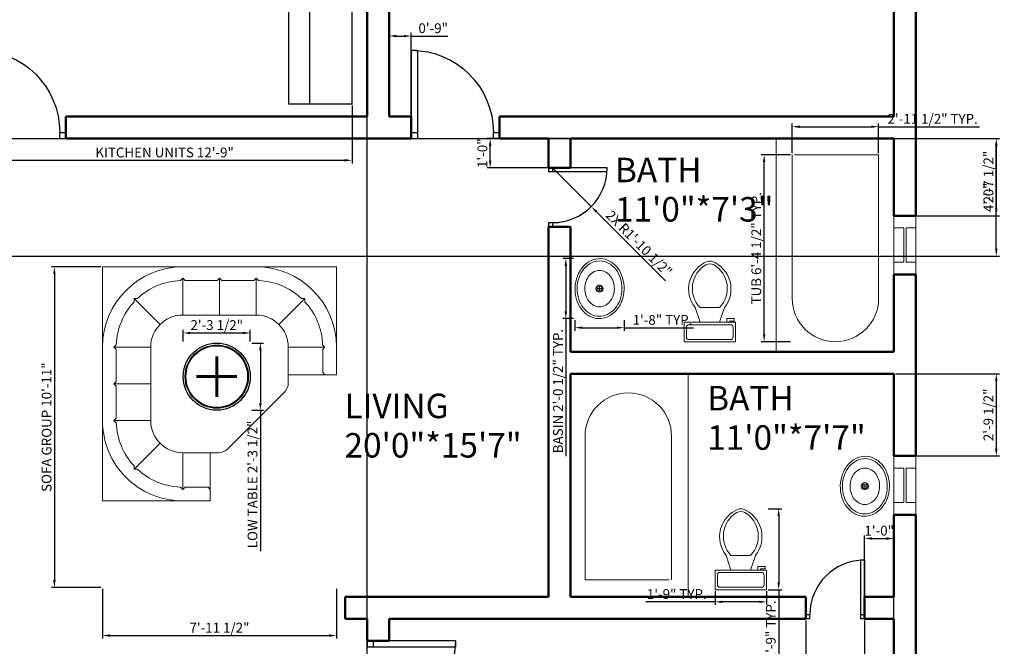
# Model space of a CAD drawing. Units: inches. Extents: x 2201 to 2875, y 1361 to 2074.
# Tile 3 of 4: x 2474 to 2875, y 1600 to 1855. Entities that reach past the tile are written whole.
import ezdxf

# ---------------------------------------------------------------- set-up
doc = ezdxf.new("R2010")
doc.units = ezdxf.units.IN
for name, color, linetype, lineweight in [('A-ANNO-DIMS', 2, 'Continuous', 18), ('A-AREA-IDEN', 7, 'Continuous', 25), ('A-FLOR-FIXT', 9, 'Continuous', 18), ('doors', 5, 'Continuous', 25), ('furniture', 8, 'Continuous', 18), ('ventilator', 3, 'Continuous', 18), ('walls', 6, 'Continuous', 50)]:
    doc.layers.add(name, color=color, linetype=linetype, lineweight=lineweight)
doc.layers.add('TEFRIŞ', color=11, linetype='Continuous')
doc.styles.get("Standard").update_dxf_attribs({"font": 'arial.ttf'})
doc.dimstyles.new('ISO-25', dxfattribs={"dimtxt": 4, "dimasz": 3, "dimexe": 1.25, "dimexo": 0.625, "dimtad": 1, "dimlunit": 3, "dimtxsty": 'Standard', "dimcen": 2.5, "dimadec": 0, "dimazin": 0, "dimtfac": 1, "dimtmove": 0, "dimatfit": 3, "dimfxl": 1, "dimarcsym": 0})

# ---------------------------------------------------------------- blocks, each defined once
blk = doc.blocks.new('12PRST09')
at = {"color": 0, "linetype": 'ByBlock'}
for p, q in [((47, 102), (0, 102)), ((0, 102), (0, 0)), ((47, 102), (47, 81)), ((35, 97), (33.98, 95.98)), ((36, 96), (35, 97)), ((35, 81), (35, 97)), ((36, 96), (46, 96)), ((46, 96), (47, 97)), ((15.23, 88.21), (13.79, 88.21)), ((13.79, 88.21), (13.79, 86.77)), ((25.1, 76.9), (13.79, 88.21)), ((50.51, 81), (35, 81)), ((54.76, 79.24), (79.24, 54.76)), ((5, 67), (6.02, 68.02)), ((6, 66), (5, 67)), ((21, 67), (5, 67)), ((6, 52), (6, 66)), ((21, 67), (21, 35)), ((5, 51), (6, 52)), ((6, 50), (5, 51)), ((21, 51), (5, 51)), ((6, 36), (6, 50)), ((81, 35), (81, 50.51)), ((102, 47), (81, 47)), ((96, 46), (97, 47)), ((96, 36), (96, 46)), ((102, 0), (102, 47)), ((6, 36), (5, 35)), ((21, 35), (5, 35)), ((5, 35), (6.02, 33.98)), ((81, 35), (97, 35)), ((97, 35), (95.98, 33.98)), ((96, 36), (97, 35)), ((25.1, 25.1), (13.79, 13.79)), ((76.9, 25.1), (88.21, 13.79)), ((35, 21), (35, 5)), ((35, 21), (67, 21)), ((51, 21), (51, 5)), ((67, 21), (67, 5)), ((13.79, 13.79), (13.79, 15.23)), ((15.23, 13.79), (13.79, 13.79)), ((86.77, 13.79), (88.21, 13.79)), ((88.21, 13.79), (88.21, 15.23)), ((35, 5), (33.98, 6.02)), ((36, 6), (35, 5)), ((50, 6), (36, 6)), ((50, 6), (51, 5)), ((51, 5), (52, 6)), ((66, 6), (52, 6)), ((66, 6), (67, 5)), ((67, 5), (68.02, 6.02)), ((0, 0), (102, 0))]:
    blk.add_line(p, q, dxfattribs=at)
for centre, radius, start, end in [((35, 67), 35, 90, 180), ((35, 67), 29, 92.0114, 132.9886), ((35, 67), 29, 137.0114, 177.9886), ((35, 67), 14, 90, 180), ((50.51, 75), 6, 45, 90), ((75, 50.51), 6, 0, 45), ((35, 35), 35, 180, 270), ((35, 35), 14, 180, 270), ((67, 35), 14, 270, 0), ((67, 35), 35, 270, 0), ((35, 35), 29, 182.0114, 222.9886), ((67, 35), 29, 317.0114, 357.9886), ((35, 35), 29, 227.0114, 267.9886), ((67, 35), 29, 272.0114, 312.9886)]:
    blk.add_arc(centre, radius, start, end, dxfattribs=at)
for tag, p, flags in [('ITEM', (75, 96), 3), ('ROOM_NUMBER', (74, 86), 1), ('DEPTH', (75, 74), 3), ('WIDTH', (75, 65), 3)]:
    blk.add_attdef(tag, p, '', height=6, dxfattribs=dict(at, flags=flags))
blk = doc.blocks.new('31')
at = {"layer": 'TEFRIŞ'}
for p, q in [((-1268.3, -203.6), (-1268.3, -264.3)), ((-1268.3, -264.3), (-1268.3, -203.6)), ((-1268.3, -264.3), (-1268.3, -203.6)), ((-1268.3, -203.6), (-1268.3, -264.3)), ((-1267.3, -203.6), (-1267.3, -264.3)), ((-1267.3, -264.3), (-1267.3, -203.6)), ((-1267.3, -264.3), (-1267.3, -203.6)), ((-1267.3, -203.6), (-1267.3, -264.3)), ((-1266.3, -203.6), (-1266.3, -264.3)), ((-1266.3, -264.3), (-1266.3, -203.6)), ((-1266.3, -264.3), (-1266.3, -203.6)), ((-1266.3, -203.6), (-1266.3, -264.3)), ((-1297.6, -232.9), (-1237, -232.9)), ((-1237, -232.9), (-1297.6, -232.9)), ((-1237, -232.9), (-1297.6, -232.9)), ((-1297.6, -232.9), (-1237, -232.9)), ((-1297.6, -233.9), (-1237, -233.9)), ((-1237, -233.9), (-1297.6, -233.9)), ((-1237, -233.9), (-1297.6, -233.9)), ((-1297.6, -233.9), (-1237, -233.9)), ((-1297.6, -234.9), (-1237, -234.9)), ((-1237, -234.9), (-1297.6, -234.9)), ((-1237, -234.9), (-1297.6, -234.9)), ((-1297.6, -234.9), (-1237, -234.9))]:
    blk.add_line(p, q, dxfattribs=at)
for radius in [50.3, 47.3, 46.3]:
    blk.add_circle((-1267.3, -233.9), radius, dxfattribs=at)
blk = doc.blocks.new('A$C008029BD')
at = {"layer": 'TEFRIŞ', "ltscale": 0.05}
for p, q in [((0, 0), (0, -3.55)), ((3.3699, 0), (0, 0)), ((3.3699, 0), (3.3699, -0.6)), ((1.5225, -0.4), (0, -0.4)), ((3.3699, -0.4), (2.0825, -0.4)), ((0.05, -0.5806), (0.05, -1.8694)), ((0.05, -0.5806), (0.55, -0.5806)), ((0.096, -0.6166), (0.454, -0.6166)), ((0.55, -0.5806), (0.55, -1.8694)), ((0.6, -2.71), (0.6, -0.6)), ((3.3699, -0.6), (0.6, -0.6)), ((0.086, -1.7734), (0.086, -0.6766)), ((0.0991, -0.6595), (0.4571, -0.6595)), ((0.1131, -0.954), (0.1131, -0.6955)), ((0.4931, -0.6955), (0.4931, -0.954)), ((0.514, -0.6766), (0.514, -1.7734)), ((0.2301, -0.8457), (0.2288, -0.9671)), ((0.2801, -0.8455), (0.2768, -1.1584)), ((0.096, -1.0242), (0.454, -1.0242)), ((0.4571, -0.99), (0.0991, -0.99)), ((0.2282, -1.0198), (0.2268, -1.1586)), ((0.11, -1.3187), (0.11, -1.0602)), ((0.49, -1.0602), (0.49, -1.3187)), ((0.454, -1.3547), (0.096, -1.3547)), ((0.096, -1.3912), (0.454, -1.3912)), ((0.11, -1.7734), (0.11, -1.4272)), ((0.1544, -1.7734), (0.1544, -1.4272)), ((0.2144, -1.7734), (0.2144, -1.4272)), ((0.2744, -1.7734), (0.2744, -1.4272)), ((0.3344, -1.7734), (0.3344, -1.4272)), ((0.3902, -1.7734), (0.3902, -1.4272)), ((0.4444, -1.7734), (0.4444, -1.4272)), ((0.49, -1.4272), (0.49, -1.7734)), ((0.454, -1.8094), (0.096, -1.8094)), ((0.454, -1.8334), (0.096, -1.8334)), ((0.55, -1.8694), (0.05, -1.8694)), ((0, -2.025), (0.4, -2.025)), ((0.4, -2.71), (0.4, -2.025)), ((0, -2.71), (0.6, -2.71)), ((0, -3.55), (0.65, -3.55))]:
    blk.add_line(p, q, dxfattribs=at)
at = {"layer": 'TEFRIŞ'}
blk.add_line((1.9688, -0.05), (1.9688, -0.5719), dxfattribs=at)
at = {"layer": 'TEFRIŞ', "ltscale": 0.05}
for points in [[(1.5225, -0.05), (2.0825, -0.05), (2.0825, -0.5719), (1.5225, -0.5719)], [(0.67, -2.73), (0.67, -3.53), (0.07, -3.53), (0.07, -2.73)], [(0.72, -2.78), (0.72, -3.48), (0.67, -3.48), (0.67, -2.78)]]:
    blk.add_lwpolyline(points, close=True, dxfattribs=at)
at = {"layer": 'TEFRIŞ', "const_width": 0.025}
for points in [[(2.0136, -0.1231, 1), (2.0386, -0.1231, 1)], [(2.0136, -0.2361, 1), (2.0386, -0.2361, 1)], [(2.0136, -0.3269, 1), (2.0386, -0.3269, 1)], [(2.0136, -0.4399, 1), (2.0386, -0.4399, 1)]]:
    blk.add_lwpolyline(points, format="xyb", close=True, dxfattribs=at)
at = {"layer": 'TEFRIŞ', "ltscale": 0.05}
for centre, radius in [((1.6277, -0.1636), 0.0505), ((1.6277, -0.4499), 0.0505), ((0.255, -0.8197), 0.036), ((0.2519, -1.1844), 0.036)]:
    blk.add_circle(centre, radius, dxfattribs=at)
at = {"layer": 'TEFRIŞ'}
for centre in [(1.8804, -0.1636), (1.8804, -0.4499)]:
    blk.add_circle(centre, 0.0505, dxfattribs=at)
at = {"layer": 'TEFRIŞ', "ltscale": 0.05}
for centre, radius, start, end in [((0.1083, -0.6495), 0.0351, 110.49764, 230.57771), ((0.454, -0.6766), 0.06, 0, 90), ((0.1177, -0.673), 0.023, 143.98534, 258.51568), ((0.4571, -0.6955), 0.036, 0, 90), ((0.1146, -1.0377), 0.023, 143.98534, 258.51568), ((0.1177, -0.9765), 0.023, 101.48432, 216.01466), ((0.454, -1.0602), 0.036, 0, 90), ((0.4571, -0.954), 0.036, 270, 0), ((0.1146, -1.3412), 0.023, 101.48432, 216.01466), ((0.1146, -1.4047), 0.023, 143.98534, 258.51568), ((0.454, -1.3187), 0.036, 270, 0), ((0.454, -1.4272), 0.036, 0, 90), ((0.1083, -1.8005), 0.0351, 129.42229, 249.50236), ((0.1146, -1.7959), 0.023, 101.48432, 216.01466), ((0.454, -1.7734), 0.06, 270, 0), ((0.454, -1.7734), 0.036, 270, 0)]:
    blk.add_arc(centre, radius, start, end, dxfattribs=at)
blk = doc.blocks.new('Sink - Oval top')
for p, q in [((-1, 0), (1, 0)), ((0, 1), (0, -1))]:
    blk.add_line(p, q)
for points in [[(-12.23, 0.39, 0.117634), (-11.46, -3.36, 0.104469), (-8.88, -6.8, 0.090016), (-5.08, -9.07, 0.08192), (-0.32, -10.02, 0.08192), (4.49, -9.38, 0.090016), (8.42, -7.36, 0.104469), (11.22, -4.09, 0.117634), (12.23, -0.39, 0.117634), (11.46, 3.36, 0.104469), (8.88, 6.8, 0.090016), (5.08, 9.07, 0.08192), (0.32, 10.02, 0.08192), (-4.49, 9.38, 0.090016), (-8.42, 7.36, 0.104469), (-11.22, 4.09, 0.117634)], [(-11.29, 0.16, 0.118622), (-10.52, -3.25, 0.104678), (-8.07, -6.36, 0.089562), (-4.54, -8.37, 0.081185), (-0.13, -9.15, 0.081185), (4.3, -8.49, 0.089562), (7.89, -6.58, 0.104678), (10.42, -3.55, 0.118622), (11.29, -0.16, 0.118622), (10.52, 3.25, 0.104678), (8.07, 6.36, 0.089562), (4.54, 8.37, 0.081185), (0.13, 9.15, 0.081185), (-4.3, 8.49, 0.089562), (-7.89, 6.58, 0.104678), (-10.42, 3.55, 0.118622)], [(-7.42, 0.08, 0.118283), (-6.91, -2.17, 0.104607), (-5.29, -4.21, 0.089718), (-2.97, -5.53, 0.081436), (-0.07, -6.04, 0.081436), (2.84, -5.59, 0.089718), (5.2, -4.33, 0.104607), (6.86, -2.32, 0.118283), (7.42, -0.08, 0.118283), (6.91, 2.17, 0.104607), (5.29, 4.21, 0.089718), (2.97, 5.53, 0.081436), (0.07, 6.04, 0.081436), (-2.84, 5.59, 0.089718), (-5.2, 4.33, 0.104607), (-6.86, 2.32, 0.118283)]]:
    blk.add_lwpolyline(points, format="xyb", close=True)
for radius in [1.5, 1]:
    blk.add_circle((0, 0), radius)
blk = doc.blocks.new('Toilet - top')
for p, q in [((9.5, -6), (9.5, -2)), ((-8, -8.5), (-8, -8)), ((-7, -8), (-7, -9.5)), ((-4, -8), (-6, -14)), ((4, -8), (6, -14)), ((-10, -8.5), (-8, -8.5)), ((-10, -9.5), (-10, -8.5)), ((-7, -9.5), (-10, -9.5)), ((4, -14), (-4, -14))]:
    blk.add_line(p, q)
blk.add_lwpolyline([(10.5, -8), (10.5, 0), (-10.5, 0), (-10.5, -8)], close=True)
for points in [[(-9.5, -2), (-9.5, -6)], [(8.5, -1), (-8.5, -1)], [(-8.5, -7), (8.5, -7)]]:
    blk.add_lwpolyline(points)
for centre, radius, start, end in [((-8.62, -1.88), 0.884, 81.8699, 188.1301), ((8.62, -1.88), 0.884, 351.8699, 98.1301), ((-8.62, -6.12), 0.884, 171.8699, 278.1301), ((8.62, -6.12), 0.884, 261.8699, 8.1301), ((3.52, -21.58), 12.17, 141.4691, 247.9714), ((4.2, -21.82), 11.33, 136.3677, 238.9468), ((-3.52, -21.58), 12.17, 292.0284, 38.5307), ((-4.2, -21.82), 11.33, 301.053, 43.6321), ((0, -27.88), 4, 245.7318, 294.2682), ((0, -29), 4, 254.8605, 285.1395)]:
    blk.add_arc(centre, radius, start, end)
blk = doc.blocks.new('DOOR-SWING-36IN')
for p, q in [((33.5, 36), (33.5, 0)), ((36, 36), (33.5, 36)), ((36, 36), (36, 0)), ((2.5, 2.5), (0, 2.5)), ((0, 0), (0, 2.5)), ((2.5, 0), (2.5, 2.5)), ((36, 2.5), (33.5, 2.5)), ((2.5, 0), (0, 0)), ((36, 0), (33.5, 0))]:
    blk.add_line(p, q)
blk.add_arc((36, 2.5), 33.5, 90, 180)
blk = doc.blocks.new('VENT-24IN')
for p, q in [((0, 24), (0, 0)), ((9, 24), (0, 24)), ((9, 0), (9, 24)), ((4, 19), (0, 19)), ((4, 19), (4, 5)), ((9, 19), (5, 19)), ((5, 19), (5, 5)), ((0, 5), (4, 5)), ((5, 5), (9, 5)), ((0, 0), (9, 0))]:
    blk.add_line(p, q)
blk = doc.blocks.new('BATH-TUB')
blk.add_lwpolyline([(0, 76.27), (0, 17.65, 1), (35.29, 17.65), (35.29, 76.27), (0.92, 76.27)], format="xyb")
blk = doc.blocks.new('*D24')
at = {"layer": 'A-ANNO-DIMS', "color": 0, "lineweight": -2, "transparency": 16777216}
for p, q in [((2699.56, 1757.92), (2695.25, 1757.92)), ((2696.5, 1754.92), (2696.5, 1736.37)), ((2699.56, 1733.37), (2695.25, 1733.37)), ((2696.5, 1733.37), (2696.5, 1677.27))]:
    blk.add_line(p, q, dxfattribs=at)
at = {"layer": 'A-ANNO-DIMS', "color": 0, "transparency": 16777216}
for points in [[(2696, 1754.92), (2697, 1754.92), (2696.5, 1757.92)], [(2696, 1736.37), (2697, 1736.37), (2696.5, 1733.37)]]:
    blk.add_solid(points, dxfattribs=at)
at = {"layer": 'Defpoints', "color": 0, "transparency": 16777216}
for p in [(2700.19, 1757.92), (2696.5, 1733.37), (2700.19, 1733.37)]:
    blk.add_point(p, dxfattribs=at)
at = {"layer": 'A-ANNO-DIMS', "color": 0, "transparency": 16777216, "insert": (2693.81, 1703.82), "char_height": 4, "attachment_point": 5, "rotation": 90}
blk.add_mtext('BASIN 2\'-0 1/2" TYP.', dxfattribs=at)
blk = doc.blocks.new('*D25')
at = {"layer": 'A-ANNO-DIMS', "color": 0, "lineweight": -2, "transparency": 16777216}
for p, q in [((2700.19, 1732.74), (2700.19, 1728.44)), ((2720.32, 1732.74), (2720.32, 1728.44)), ((2703.19, 1729.69), (2717.32, 1729.69)), ((2720.32, 1729.69), (2748.58, 1729.69))]:
    blk.add_line(p, q, dxfattribs=at)
at = {"layer": 'A-ANNO-DIMS', "color": 0, "transparency": 16777216}
for points in [[(2703.19, 1730.19), (2703.19, 1729.19), (2700.19, 1729.69)], [(2717.32, 1730.19), (2717.32, 1729.19), (2720.32, 1729.69)]]:
    blk.add_solid(points, dxfattribs=at)
at = {"layer": 'Defpoints', "color": 0, "transparency": 16777216}
for p in [(2700.19, 1733.37), (2720.32, 1733.37), (2720.32, 1729.69)]:
    blk.add_point(p, dxfattribs=at)
at = {"layer": 'A-ANNO-DIMS', "color": 0, "transparency": 16777216, "insert": (2735.95, 1732.35), "char_height": 4, "attachment_point": 5}
blk.add_mtext('1\'-8" TYP.', dxfattribs=at)
blk = doc.blocks.new('*D26')
at = {"layer": 'A-ANNO-DIMS', "color": 0, "lineweight": -2, "transparency": 16777216}
for p, q in [((2779.03, 1655.83), (2784.62, 1655.83)), ((2783.37, 1652.83), (2783.37, 1625.78)), ((2779.03, 1622.78), (2784.62, 1622.78)), ((2783.37, 1622.78), (2783.37, 1583.13))]:
    blk.add_line(p, q, dxfattribs=at)
at = {"layer": 'A-ANNO-DIMS', "color": 0, "transparency": 16777216}
for points in [[(2782.87, 1652.83), (2783.87, 1652.83), (2783.37, 1655.83)], [(2782.87, 1625.78), (2783.87, 1625.78), (2783.37, 1622.78)]]:
    blk.add_solid(points, dxfattribs=at)
at = {"layer": 'Defpoints', "color": 0, "transparency": 16777216}
for p in [(2778.41, 1655.83), (2778.41, 1622.78), (2783.37, 1622.78)]:
    blk.add_point(p, dxfattribs=at)
at = {"layer": 'A-ANNO-DIMS', "color": 0, "transparency": 16777216, "insert": (2780.67, 1601.46), "char_height": 4, "attachment_point": 5, "rotation": 90}
blk.add_mtext('WC 2\'-9" TYP.', dxfattribs=at)
blk = doc.blocks.new('*D27')
at = {"layer": 'A-ANNO-DIMS', "color": 0, "lineweight": -2, "transparency": 16777216}
for p, q in [((2757.41, 1622.16), (2757.41, 1616.58)), ((2778.41, 1622.16), (2778.41, 1616.58)), ((2757.41, 1617.83), (2729.15, 1617.83)), ((2775.41, 1617.83), (2760.41, 1617.83))]:
    blk.add_line(p, q, dxfattribs=at)
at = {"layer": 'A-ANNO-DIMS', "color": 0, "transparency": 16777216}
for points in [[(2760.41, 1618.33), (2760.41, 1617.33), (2757.41, 1617.83)], [(2775.41, 1618.33), (2775.41, 1617.33), (2778.41, 1617.83)]]:
    blk.add_solid(points, dxfattribs=at)
at = {"layer": 'Defpoints', "color": 0, "transparency": 16777216}
for p in [(2757.41, 1622.78), (2778.41, 1622.78), (2757.41, 1617.83)]:
    blk.add_point(p, dxfattribs=at)
at = {"layer": 'A-ANNO-DIMS', "color": 0, "transparency": 16777216, "insert": (2741.78, 1620.49), "char_height": 4, "attachment_point": 5}
blk.add_mtext('1\'-9" TYP.', dxfattribs=at)
blk = doc.blocks.new('*D28')
at = {"layer": 'A-ANNO-DIMS', "color": 0, "lineweight": -2, "transparency": 16777216}
for p, q in [((2788.25, 1800.25), (2776.19, 1800.25)), ((2777.44, 1726.98), (2777.44, 1797.25)), ((2788.25, 1723.98), (2776.19, 1723.98))]:
    blk.add_line(p, q, dxfattribs=at)
at = {"layer": 'A-ANNO-DIMS', "color": 0, "transparency": 16777216}
for points in [[(2776.94, 1797.25), (2777.94, 1797.25), (2777.44, 1800.25)], [(2776.94, 1726.98), (2777.94, 1726.98), (2777.44, 1723.98)]]:
    blk.add_solid(points, dxfattribs=at)
at = {"layer": 'Defpoints', "color": 0, "transparency": 16777216}
for p in [(2777.44, 1800.25), (2788.88, 1800.25), (2788.88, 1723.98)]:
    blk.add_point(p, dxfattribs=at)
at = {"layer": 'A-ANNO-DIMS', "color": 0, "transparency": 16777216, "insert": (2774.74, 1762.11), "char_height": 4, "attachment_point": 5, "rotation": 90}
blk.add_mtext('TUB 6\'-4 1/2" TYP.', dxfattribs=at)
blk = doc.blocks.new('*D29')
at = {"layer": 'A-ANNO-DIMS', "color": 0, "lineweight": -2, "transparency": 16777216}
for p, q in [((2788.88, 1800.87), (2788.88, 1812.94)), ((2824.17, 1800.87), (2824.17, 1812.94)), ((2791.88, 1811.69), (2821.17, 1811.69)), ((2824.17, 1811.69), (2865.3, 1811.69))]:
    blk.add_line(p, q, dxfattribs=at)
at = {"layer": 'A-ANNO-DIMS', "color": 0, "transparency": 16777216}
for points in [[(2791.88, 1812.19), (2791.88, 1811.19), (2788.88, 1811.69)], [(2821.17, 1812.19), (2821.17, 1811.19), (2824.17, 1811.69)]]:
    blk.add_solid(points, dxfattribs=at)
at = {"layer": 'Defpoints', "color": 0, "transparency": 16777216}
for p in [(2824.17, 1811.69), (2788.88, 1800.25), (2824.17, 1800.25)]:
    blk.add_point(p, dxfattribs=at)
at = {"layer": 'A-ANNO-DIMS', "color": 0, "transparency": 16777216, "insert": (2846.23, 1814.38), "char_height": 4, "attachment_point": 5}
blk.add_mtext('2\'-11 1/2" TYP.', dxfattribs=at)
blk = doc.blocks.new('*D30')
at = {"layer": 'A-ANNO-DIMS', "color": 0, "lineweight": -2, "transparency": 16777216}
for p, q in [((2506.74, 1754.52), (2486.49, 1754.52)), ((2487.74, 1751.52), (2487.74, 1626.7)), ((2506.74, 1623.7), (2486.49, 1623.7))]:
    blk.add_line(p, q, dxfattribs=at)
at = {"layer": 'A-ANNO-DIMS', "color": 0, "transparency": 16777216}
for points in [[(2487.24, 1751.52), (2488.24, 1751.52), (2487.74, 1754.52)], [(2487.24, 1626.7), (2488.24, 1626.7), (2487.74, 1623.7)]]:
    blk.add_solid(points, dxfattribs=at)
at = {"layer": 'Defpoints', "color": 0, "transparency": 16777216}
for p in [(2507.37, 1754.52), (2487.74, 1623.7), (2507.37, 1623.7)]:
    blk.add_point(p, dxfattribs=at)
at = {"layer": 'A-ANNO-DIMS', "color": 0, "transparency": 16777216, "insert": (2485.05, 1689.11), "char_height": 4, "attachment_point": 5, "rotation": 90}
blk.add_mtext('SOFA GROUP 10\'-11"', dxfattribs=at)
blk = doc.blocks.new('*D31')
at = {"layer": 'A-ANNO-DIMS', "color": 0, "lineweight": -2, "transparency": 16777216}
for p, q in [((2507.37, 1623.08), (2507.37, 1602.83)), ((2602.85, 1623.08), (2602.85, 1602.83)), ((2510.37, 1604.08), (2599.85, 1604.08))]:
    blk.add_line(p, q, dxfattribs=at)
at = {"layer": 'A-ANNO-DIMS', "color": 0, "transparency": 16777216}
for points in [[(2510.37, 1604.58), (2510.37, 1603.58), (2507.37, 1604.08)], [(2599.85, 1604.58), (2599.85, 1603.58), (2602.85, 1604.08)]]:
    blk.add_solid(points, dxfattribs=at)
at = {"layer": 'Defpoints', "color": 0, "transparency": 16777216}
for p in [(2507.37, 1623.7), (2602.85, 1623.7), (2602.85, 1604.08)]:
    blk.add_point(p, dxfattribs=at)
at = {"layer": 'A-ANNO-DIMS', "color": 0, "transparency": 16777216, "insert": (2555.11, 1606.77), "char_height": 4, "attachment_point": 5}
blk.add_mtext('7\'-11 1/2"', dxfattribs=at)
blk = doc.blocks.new('*D32')
at = {"layer": 'A-ANNO-DIMS', "color": 0, "lineweight": -2, "transparency": 16777216}
for p, q in [((2568.32, 1723.43), (2573.05, 1723.43)), ((2571.8, 1720.43), (2571.8, 1699.02)), ((2568.32, 1696.02), (2573.05, 1696.02)), ((2571.8, 1696.02), (2571.8, 1638.46))]:
    blk.add_line(p, q, dxfattribs=at)
at = {"layer": 'A-ANNO-DIMS', "color": 0, "transparency": 16777216}
for points in [[(2571.3, 1720.43), (2572.3, 1720.43), (2571.8, 1723.43)], [(2571.3, 1699.02), (2572.3, 1699.02), (2571.8, 1696.02)]]:
    blk.add_solid(points, dxfattribs=at)
at = {"layer": 'Defpoints', "color": 0, "transparency": 16777216}
for p in [(2567.69, 1723.43), (2567.69, 1696.02), (2571.8, 1696.02)]:
    blk.add_point(p, dxfattribs=at)
at = {"layer": 'A-ANNO-DIMS', "color": 0, "transparency": 16777216, "insert": (2569.11, 1665.74), "char_height": 4, "attachment_point": 5, "rotation": 90}
blk.add_mtext('LOW TABLE 2\'-3 1/2"', dxfattribs=at)
blk = doc.blocks.new('*D33')
at = {"layer": 'A-ANNO-DIMS', "color": 0, "lineweight": -2, "transparency": 16777216}
for p, q in [((2540.28, 1724.06), (2540.28, 1728.79)), ((2567.69, 1724.06), (2567.69, 1728.79)), ((2543.28, 1727.54), (2564.69, 1727.54))]:
    blk.add_line(p, q, dxfattribs=at)
at = {"layer": 'A-ANNO-DIMS', "color": 0, "transparency": 16777216}
for points in [[(2543.28, 1728.04), (2543.28, 1727.04), (2540.28, 1727.54)], [(2564.69, 1728.04), (2564.69, 1727.04), (2567.69, 1727.54)]]:
    blk.add_solid(points, dxfattribs=at)
at = {"layer": 'Defpoints', "color": 0, "transparency": 16777216}
for p in [(2567.69, 1727.54), (2540.28, 1723.43), (2567.69, 1723.43)]:
    blk.add_point(p, dxfattribs=at)
at = {"layer": 'A-ANNO-DIMS', "color": 0, "transparency": 16777216, "insert": (2553.99, 1730.24), "char_height": 4, "attachment_point": 5}
blk.add_mtext('2\'-3 1/2"', dxfattribs=at)
blk = doc.blocks.new('*D34')
at = {"layer": 'A-ANNO-DIMS', "color": 0, "lineweight": -2, "transparency": 16777216}
for p, q in [((2456.14, 1820.31), (2456.14, 1796.72)), ((2609.26, 1820.31), (2609.26, 1796.72)), ((2459.14, 1797.97), (2606.26, 1797.97))]:
    blk.add_line(p, q, dxfattribs=at)
at = {"layer": 'A-ANNO-DIMS', "color": 0, "transparency": 16777216}
for points in [[(2459.14, 1798.47), (2459.14, 1797.47), (2456.14, 1797.97)], [(2606.26, 1798.47), (2606.26, 1797.47), (2609.26, 1797.97)]]:
    blk.add_solid(points, dxfattribs=at)
at = {"layer": 'Defpoints', "color": 0, "transparency": 16777216}
for p in [(2456.14, 1820.94), (2609.26, 1820.94), (2609.26, 1797.97)]:
    blk.add_point(p, dxfattribs=at)
at = {"layer": 'A-ANNO-DIMS', "color": 0, "transparency": 16777216, "insert": (2532.7, 1800.66), "char_height": 4, "attachment_point": 5}
blk.add_mtext('KITCHEN UNITS 12\'-9"', dxfattribs=at)
blk = doc.blocks.new('*D40')
at = {"layer": 'A-ANNO-DIMS', "color": 0, "lineweight": -2, "transparency": 16777216}
for p, q in [((2831.03, 1806.88), (2873.45, 1806.88)), ((2872.2, 1803.88), (2872.2, 1778.38)), ((2831.03, 1775.38), (2873.45, 1775.38))]:
    blk.add_line(p, q, dxfattribs=at)
at = {"layer": 'A-ANNO-DIMS', "color": 0, "transparency": 16777216}
for points in [[(2871.7, 1803.88), (2872.7, 1803.88), (2872.2, 1806.88)], [(2871.7, 1778.38), (2872.7, 1778.38), (2872.2, 1775.38)]]:
    blk.add_solid(points, dxfattribs=at)
at = {"layer": 'Defpoints', "color": 0, "transparency": 16777216}
for p in [(2830.4, 1806.88), (2830.4, 1775.38), (2872.2, 1775.38)]:
    blk.add_point(p, dxfattribs=at)
at = {"layer": 'A-ANNO-DIMS', "color": 0, "transparency": 16777216, "insert": (2869.51, 1791.13), "char_height": 4, "attachment_point": 5, "rotation": 90}
blk.add_mtext('2\'-7 1/2"', dxfattribs=at)
blk = doc.blocks.new('*D41')
at = {"layer": 'A-ANNO-DIMS', "color": 0, "lineweight": -2, "transparency": 16777216}
for p, q in [((2831.03, 1710.88), (2873.45, 1710.88)), ((2872.2, 1707.88), (2872.2, 1680.38)), ((2831.03, 1677.38), (2873.45, 1677.38))]:
    blk.add_line(p, q, dxfattribs=at)
at = {"layer": 'A-ANNO-DIMS', "color": 0, "transparency": 16777216}
for points in [[(2871.7, 1707.88), (2872.7, 1707.88), (2872.2, 1710.88)], [(2871.7, 1680.38), (2872.7, 1680.38), (2872.2, 1677.38)]]:
    blk.add_solid(points, dxfattribs=at)
at = {"layer": 'Defpoints', "color": 0, "transparency": 16777216}
for p in [(2830.4, 1710.88), (2830.4, 1677.38), (2872.2, 1677.38)]:
    blk.add_point(p, dxfattribs=at)
at = {"layer": 'A-ANNO-DIMS', "color": 0, "transparency": 16777216, "insert": (2869.51, 1694.13), "char_height": 4, "attachment_point": 5, "rotation": 90}
blk.add_mtext('2\'-9 1/2"', dxfattribs=at)
blk = doc.blocks.new('*D47')
at = {"layer": 'A-ANNO-DIMS', "color": 0, "lineweight": -2, "transparency": 16777216}
for p, q in [((2794.4, 1610.26), (2794.4, 1576.83)), ((2818.4, 1610.26), (2818.4, 1576.83)), ((2815.4, 1578.08), (2797.4, 1578.08))]:
    blk.add_line(p, q, dxfattribs=at)
at = {"layer": 'A-ANNO-DIMS', "color": 0, "transparency": 16777216}
for points in [[(2797.4, 1578.58), (2797.4, 1577.58), (2794.4, 1578.08)], [(2815.4, 1578.58), (2815.4, 1577.58), (2818.4, 1578.08)]]:
    blk.add_solid(points, dxfattribs=at)
at = {"layer": 'Defpoints', "color": 0, "transparency": 16777216}
for p in [(2794.4, 1610.88), (2818.4, 1610.88), (2794.4, 1578.08)]:
    blk.add_point(p, dxfattribs=at)
at = {"layer": 'A-ANNO-DIMS', "color": 0, "transparency": 16777216, "insert": (2806.4, 1580.75), "char_height": 4, "attachment_point": 5}
blk.add_mtext('2\'-0"', dxfattribs=at)
blk = doc.blocks.new('*D48')
at = {"layer": 'A-ANNO-DIMS', "color": 0, "lineweight": -2, "transparency": 16777216}
for p, q in [((2818.4, 1611.51), (2818.4, 1644.93)), ((2830.4, 1611.51), (2830.4, 1644.93)), ((2821.4, 1643.68), (2827.4, 1643.68))]:
    blk.add_line(p, q, dxfattribs=at)
at = {"layer": 'A-ANNO-DIMS', "color": 0, "transparency": 16777216}
for points in [[(2821.4, 1644.18), (2821.4, 1643.18), (2818.4, 1643.68)], [(2827.4, 1644.18), (2827.4, 1643.18), (2830.4, 1643.68)]]:
    blk.add_solid(points, dxfattribs=at)
at = {"layer": 'Defpoints', "color": 0, "transparency": 16777216}
for p in [(2830.4, 1643.68), (2818.4, 1610.88), (2830.4, 1610.88)]:
    blk.add_point(p, dxfattribs=at)
at = {"layer": 'A-ANNO-DIMS', "color": 0, "transparency": 16777216, "insert": (2824.4, 1646.35), "char_height": 4, "attachment_point": 5}
blk.add_mtext('1\'-0"', dxfattribs=at)
blk = doc.blocks.new('*D50')
at = {"layer": 'A-ANNO-DIMS', "color": 0, "lineweight": -2, "transparency": 16777216}
for p, q in [((2365.03, 1806.88), (2873.45, 1806.88)), ((2872.2, 1761.88), (2872.2, 1803.88)), ((2365.03, 1758.88), (2873.45, 1758.88))]:
    blk.add_line(p, q, dxfattribs=at)
at = {"layer": 'A-ANNO-DIMS', "color": 0, "transparency": 16777216}
for points in [[(2871.7, 1803.88), (2872.7, 1803.88), (2872.2, 1806.88)], [(2871.7, 1761.88), (2872.7, 1761.88), (2872.2, 1758.88)]]:
    blk.add_solid(points, dxfattribs=at)
at = {"layer": 'Defpoints', "color": 0, "transparency": 16777216}
for p in [(2364.4, 1806.88), (2872.2, 1806.88), (2364.4, 1758.88)]:
    blk.add_point(p, dxfattribs=at)
at = {"layer": 'A-ANNO-DIMS', "color": 0, "transparency": 16777216, "insert": (2869.54, 1782.88), "char_height": 4, "attachment_point": 5, "rotation": 90}
blk.add_mtext('4\'-0"', dxfattribs=at)
blk = doc.blocks.new('*D53')
at = {"layer": 'A-ANNO-DIMS', "color": 0, "lineweight": -2, "transparency": 16777216}
for p, q in [((2624.4, 1816.51), (2624.4, 1849.93)), ((2633.4, 1816.51), (2633.4, 1849.93)), ((2627.4, 1848.68), (2630.4, 1848.68)), ((2633.4, 1848.68), (2648.29, 1848.68))]:
    blk.add_line(p, q, dxfattribs=at)
at = {"layer": 'A-ANNO-DIMS', "color": 0, "transparency": 16777216}
for points in [[(2627.4, 1849.18), (2627.4, 1848.18), (2624.4, 1848.68)], [(2630.4, 1849.18), (2630.4, 1848.18), (2633.4, 1848.68)]]:
    blk.add_solid(points, dxfattribs=at)
at = {"layer": 'Defpoints', "color": 0, "transparency": 16777216}
for p in [(2633.4, 1848.68), (2624.4, 1815.88), (2633.4, 1815.88)]:
    blk.add_point(p, dxfattribs=at)
at = {"layer": 'A-ANNO-DIMS', "color": 0, "transparency": 16777216, "insert": (2642.34, 1851.35), "char_height": 4, "attachment_point": 5}
blk.add_mtext('0\'-9"', dxfattribs=at)
blk = doc.blocks.new('*D55')
at = {"layer": 'A-ANNO-DIMS', "color": 0, "lineweight": -2, "transparency": 16777216}
for p, q in [((2697.78, 1806.88), (2664.35, 1806.88)), ((2665.6, 1797.88), (2665.6, 1803.88)), ((2697.78, 1794.88), (2664.35, 1794.88))]:
    blk.add_line(p, q, dxfattribs=at)
at = {"layer": 'A-ANNO-DIMS', "color": 0, "transparency": 16777216}
for points in [[(2665.1, 1803.88), (2666.1, 1803.88), (2665.6, 1806.88)], [(2665.1, 1797.88), (2666.1, 1797.88), (2665.6, 1794.88)]]:
    blk.add_solid(points, dxfattribs=at)
at = {"layer": 'Defpoints', "color": 0, "transparency": 16777216}
for p in [(2665.6, 1806.88), (2698.4, 1806.88), (2698.4, 1794.88)]:
    blk.add_point(p, dxfattribs=at)
at = {"layer": 'A-ANNO-DIMS', "color": 0, "transparency": 16777216, "insert": (2662.94, 1800.88), "char_height": 4, "attachment_point": 5, "rotation": 90}
blk.add_mtext('1\'-0"', dxfattribs=at)
blk = doc.blocks.new('*D56')
at = {"layer": 'A-ANNO-DIMS', "color": 0, "lineweight": -2, "transparency": 16777216}
for p, q in [((2447.4, 1395.51), (2447.4, 2069.93)), ((2615.4, 1395.51), (2615.4, 2069.93)), ((2450.4, 2068.68), (2612.4, 2068.68))]:
    blk.add_line(p, q, dxfattribs=at)
at = {"layer": 'A-ANNO-DIMS', "color": 0, "transparency": 16777216}
for points in [[(2450.4, 2069.18), (2450.4, 2068.18), (2447.4, 2068.68)], [(2612.4, 2069.18), (2612.4, 2068.18), (2615.4, 2068.68)]]:
    blk.add_solid(points, dxfattribs=at)
at = {"layer": 'Defpoints', "color": 0, "transparency": 16777216}
for p in [(2615.4, 2068.68), (2447.4, 1394.88), (2615.4, 1394.88)]:
    blk.add_point(p, dxfattribs=at)
at = {"layer": 'A-ANNO-DIMS', "color": 0, "transparency": 16777216, "insert": (2531.4, 2071.35), "char_height": 4, "attachment_point": 5}
blk.add_mtext('14\'-0"', dxfattribs=at)
blk = doc.blocks.new('*D61')
at = {"layer": 'A-ANNO-DIMS', "color": 0, "lineweight": -2, "transparency": 16777216}
for p, q in [((2691.07, 1794.88), (2706.86, 1779.09)), ((2737.13, 1748.82), (2708.98, 1776.97))]:
    blk.add_line(p, q, dxfattribs=at)
at = {"layer": 'A-ANNO-DIMS', "color": 0, "transparency": 16777216}
blk.add_solid([(2709.34, 1777.32), (2708.63, 1776.62), (2706.86, 1779.09)], dxfattribs=at)
at = {"layer": 'Defpoints', "color": 0, "transparency": 16777216}
for p in [(2691.07, 1794.88), (2706.86, 1779.09)]:
    blk.add_point(p, dxfattribs=at)
at = {"layer": 'A-ANNO-DIMS', "color": 0, "transparency": 16777216, "insert": (2726.02, 1763.74), "char_height": 4, "attachment_point": 5, "rotation": 314.9983}
blk.add_mtext('2X R1\'-10 1/2"', dxfattribs=at)

msp = doc.modelspace()

# ---------------------------------------------------------------- linework, layer by layer
at = {"layer": 'A-FLOR-FIXT'}
for p, q in [((2782.403, 1806.883), (2782.403, 1719.883)), ((2782.403, 1806.883), (2782.403, 1775.383)), ((2746.403, 1710.883), (2746.403, 1619.883))]:
    msp.add_line(p, q, dxfattribs=at)
at = {"layer": 'doors'}
for p, q in [((2713.403, 1794.883), (2689.403, 1794.883)), ((2689.403, 1794.883), (2689.403, 1793.216)), ((2713.403, 1793.216), (2689.403, 1793.216)), ((2691.069, 1794.883), (2691.069, 1793.216)), ((2689.403, 1772.549), (2689.403, 1770.883)), ((2689.403, 1772.549), (2691.069, 1772.549)), ((2691.069, 1772.549), (2691.069, 1770.883)), ((2689.403, 1770.883), (2691.069, 1770.883)), ((2816.736, 1634.883), (2816.736, 1610.883)), ((2818.403, 1634.883), (2816.736, 1634.883)), ((2818.403, 1634.883), (2818.403, 1610.883)), ((2796.069, 1612.549), (2794.403, 1612.549)), ((2794.403, 1610.883), (2794.403, 1612.549)), ((2796.069, 1610.883), (2796.069, 1612.549)), ((2818.403, 1612.549), (2816.736, 1612.549)), ((2796.069, 1610.883), (2794.403, 1610.883)), ((2818.403, 1610.883), (2816.736, 1610.883))]:
    msp.add_line(p, q, dxfattribs=at)
for centre, start, end in [((2691.069, 1794.883), 270, 0), ((2818.403, 1612.549), 90, 180)]:
    msp.add_arc(centre, 22.333, start, end, dxfattribs=at)
at = {"layer": 'walls'}
for p, q in [((2624.403, 1991.883), (2624.403, 1815.883)), ((2615.403, 1971.883), (2615.403, 1815.883)), ((2830.403, 1891.383), (2830.403, 1815.883)), ((2839.403, 1891.383), (2839.403, 1775.383)), ((2492.403, 1815.883), (2615.403, 1815.883)), ((2492.403, 1815.883), (2492.403, 1806.883)), ((2624.403, 1815.883), (2633.403, 1815.883)), ((2633.403, 1815.883), (2633.403, 1806.883)), ((2669.403, 1815.883), (2830.403, 1815.883)), ((2669.403, 1815.883), (2669.403, 1806.883)), ((2492.403, 1806.883), (2633.403, 1806.883)), ((2669.403, 1806.883), (2689.403, 1806.883)), ((2689.403, 1806.883), (2689.403, 1794.883)), ((2698.403, 1806.883), (2698.403, 1794.883)), ((2698.403, 1806.883), (2830.403, 1806.883)), ((2830.403, 1806.883), (2830.403, 1775.383)), ((2689.403, 1794.883), (2698.403, 1794.883)), ((2839.403, 1775.383), (2830.403, 1775.383)), ((2689.403, 1770.883), (2698.403, 1770.883)), ((2689.403, 1770.883), (2689.403, 1619.883)), ((2698.403, 1770.883), (2698.403, 1719.883)), ((2839.403, 1751.383), (2830.403, 1751.383)), ((2830.403, 1751.383), (2830.403, 1719.883)), ((2839.403, 1751.383), (2839.403, 1677.383)), ((2698.403, 1719.883), (2830.403, 1719.883)), ((2698.403, 1710.883), (2830.403, 1710.883)), ((2698.403, 1710.883), (2698.403, 1619.883)), ((2830.403, 1710.883), (2830.403, 1677.383)), ((2839.403, 1677.383), (2830.403, 1677.383)), ((2839.403, 1653.383), (2830.403, 1653.383)), ((2830.403, 1653.383), (2830.403, 1619.883)), ((2839.403, 1653.383), (2839.403, 1537.383)), ((2606.403, 1619.883), (2689.403, 1619.883)), ((2606.403, 1619.883), (2606.403, 1610.883)), ((2698.403, 1619.883), (2794.403, 1619.883)), ((2794.403, 1619.883), (2794.403, 1610.883)), ((2818.403, 1619.883), (2830.403, 1619.883)), ((2818.403, 1619.883), (2818.403, 1610.883)), ((2606.403, 1610.883), (2615.403, 1610.883)), ((2615.403, 1610.883), (2615.403, 1601.883)), ((2624.403, 1610.883), (2624.403, 1601.883)), ((2624.403, 1610.883), (2794.403, 1610.883)), ((2818.403, 1610.883), (2830.403, 1610.883)), ((2830.403, 1610.883), (2830.403, 1537.383)), ((2615.403, 1601.883), (2624.403, 1601.883))]:
    msp.add_line(p, q, dxfattribs=at)

# ---------------------------------------------------------------- block references
at = {"layer": 'A-FLOR-FIXT', "xscale": 43.13452976200671, "yscale": 43.13452976200671, "zscale": 43.13452976200671, "rotation": 270}
msp.add_blockref('A$C008029BD', (2609.265, 1966.296), dxfattribs=at)
at = {"layer": 'A-FLOR-FIXT'}
msp.add_blockref('BATH-TUB', (2788.877, 1723.979), dxfattribs=at)
for name, p, rotation in [('Sink - Oval top', (2710.255, 1745.644), 270), ('Toilet - top', (2755.263, 1723.873), 180), ('BATH-TUB', (2739.642, 1703.081), 180), ('Sink - Oval top', (2818.553, 1664.988), 270), ('Toilet - top', (2767.91, 1622.784), 180)]:
    msp.add_blockref(name, p, dxfattribs=dict(at, rotation=rotation))
at = {"layer": 'doors', "extrusion": (0, 0, -1), "zscale": -1}
for p in [(-2492.403, 1806.883), (-2669.403, 1806.883)]:
    msp.add_blockref('DOOR-SWING-36IN', p, dxfattribs=at)
at = {"layer": 'doors', "extrusion": (0, 0, -1), "zscale": -1, "rotation": 90.00000000000063}
msp.add_blockref('DOOR-SWING-36IN', (-2615.403, 1565.883), dxfattribs=at)
at = {"layer": 'furniture', "rotation": 270}
for name, p, xscale, yscale, zscale in [('12PRST09', (2507.365, 1754.519), 0.9361400859016036, 0.9361400859016036, 0.9361400859016036), ('31', (2617.696, 1364.604), 0.2723316613531938, 0.2723316613531938, 0.2723316613531938)]:
    msp.add_blockref(name, p, dxfattribs=dict(at, xscale=xscale, yscale=yscale, zscale=zscale))
at = {"layer": 'ventilator'}
for p in [(2830.403, 1751.383), (2830.403, 1653.383)]:
    msp.add_blockref('VENT-24IN', p, dxfattribs=at)

# ---------------------------------------------------------------- texts
at = {"layer": 'A-AREA-IDEN'}
for s, p in [('BATH', (2716.528, 1789.048)), ('11\'0"*7\'3"', (2716.528, 1772.983)), ('BATH', (2754.172, 1695.935)), ('LIVING', (2606.136, 1692.772)), ('11\'0"*7\'7"', (2754.172, 1679.871)), ('20\'0"*15\'7"', (2606.136, 1676.708))]:
    msp.add_text(s, height=10, dxfattribs=at).set_placement(p)

# ---------------------------------------------------------------- dimensions: what is measured, and where the dimension line sits
at = {"layer": 'A-ANNO-DIMS'}
for base, p1, p2, picture, middle in [((2615.403, 2068.683), (2447.403, 1394.883), (2615.403, 1394.883), '*D56', (2531.403, 2071.35)), ((2633.403, 1848.683), (2624.403, 1815.883), (2633.403, 1815.883), '*D53', (2642.344, 1851.35)), ((2567.69, 1727.543), (2540.281, 1723.431), (2567.69, 1723.431), '*D33', (2553.986, 1730.237)), ((2830.403, 1643.683), (2818.403, 1610.883), (2830.403, 1610.883), '*D48', (2824.403, 1646.35)), ((2602.852, 1604.082), (2507.365, 1623.704), (2602.852, 1623.704), '*D31', (2555.108, 1606.775))]:
    dim = msp.add_linear_dim(base=base, p1=p1, p2=p2, dimstyle='ISO-25', override={"dimdec": 1, "dimlfac": 1, "dimrnd": 0, "dimzin": 1, "dimdsep": 46, "dimlunit": 4, "dimfrac": 2}, dxfattribs=at)
    dim.commit()
    dim.dimension.update_dxf_attribs({"geometry": picture, "text_midpoint": middle})
for base, p1, p2, text, picture, middle in [((2609.265, 1797.967), (2456.137, 1820.936), (2609.265, 1820.936), 'KITCHEN UNITS <>', '*D34', (2532.701, 1800.66)), ((2824.17, 1811.69), (2788.877, 1800.25), (2824.17, 1800.25), '<> TYP.', '*D29', (2846.235, 1814.384)), ((2720.323, 1729.686), (2700.186, 1733.368), (2720.323, 1733.368), '<> TYP.', '*D25', (2735.951, 1732.353))]:
    dim = msp.add_linear_dim(base=base, p1=p1, p2=p2, text=text, dimstyle='ISO-25', override={"dimdec": 1, "dimlfac": 1, "dimrnd": 0, "dimzin": 1, "dimdsep": 46, "dimlunit": 4, "dimfrac": 2}, dxfattribs=at)
    dim.commit()
    dim.dimension.update_dxf_attribs({"geometry": picture, "text_midpoint": middle})
for base, p1, p2, angle, picture, middle in [((2872.203, 1806.883), (2364.403, 1758.883), (2364.403, 1806.883), 90, '*D50', (2869.535, 1782.883)), ((2665.603, 1806.883), (2698.403, 1794.883), (2698.403, 1806.883), 90, '*D55', (2662.935, 1800.883)), ((2872.203, 1775.383), (2830.403, 1806.883), (2830.403, 1775.383), 90, '*D40', (2869.51, 1791.133)), ((2872.203, 1677.383), (2830.403, 1710.883), (2830.403, 1677.383), 90, '*D41', (2869.51, 1694.133)), ((2794.403, 1578.083), (2818.403, 1610.883), (2794.403, 1610.883), 180, '*D47', (2806.403, 1580.75))]:
    dim = msp.add_linear_dim(base=base, p1=p1, p2=p2, angle=angle, dimstyle='ISO-25', override={"dimdec": 1, "dimlfac": 1, "dimrnd": 0, "dimzin": 1, "dimdsep": 46, "dimlunit": 4, "dimfrac": 2}, dxfattribs=at)
    dim.commit()
    dim.dimension.update_dxf_attribs({"geometry": picture, "text_midpoint": middle})
for base, p1, p2, angle, text, picture, middle in [((2777.436, 1800.25), (2788.877, 1723.979), (2788.877, 1800.25), 90, 'TUB <> TYP.', '*D28', (2774.743, 1762.114)), ((2696.504, 1733.368), (2700.186, 1757.919), (2700.186, 1733.368), 270, 'BASIN <> TYP.', '*D24', (2693.811, 1703.82)), ((2487.743, 1623.704), (2507.365, 1754.519), (2507.365, 1623.704), 270, 'SOFA GROUP <>', '*D30', (2485.049, 1689.111)), ((2571.802, 1696.023), (2567.69, 1723.431), (2567.69, 1696.023), 270, 'LOW TABLE <>', '*D32', (2569.106, 1665.741)), ((2783.367, 1622.784), (2778.41, 1655.831), (2778.41, 1622.784), 270, 'WC <> TYP.', '*D26', (2780.673, 1601.456)), ((2757.41, 1617.828), (2778.41, 1622.784), (2757.41, 1622.784), 180, '<> TYP.', '*D27', (2741.782, 1620.495))]:
    dim = msp.add_linear_dim(base=base, p1=p1, p2=p2, angle=angle, text=text, dimstyle='ISO-25', override={"dimdec": 1, "dimlfac": 1, "dimrnd": 0, "dimzin": 1, "dimdsep": 46, "dimlunit": 4, "dimfrac": 2}, dxfattribs=at)
    dim.commit()
    dim.dimension.update_dxf_attribs({"geometry": picture, "text_midpoint": middle})
dim = msp.add_radius_dim(center=(2691.069, 1794.883), mpoint=(2706.861, 1779.09), text='2X <>', dimstyle='ISO-25', override={"dimdec": 1, "dimlfac": 1, "dimrnd": 0, "dimzin": 1, "dimdsep": 46, "dimlunit": 4, "dimfrac": 2}, dxfattribs=at)
dim.commit()
dim.dimension.update_dxf_attribs({"geometry": '*D61', "text_midpoint": (2726.019, 1763.739)})

doc.saveas('drawing.dxf')
